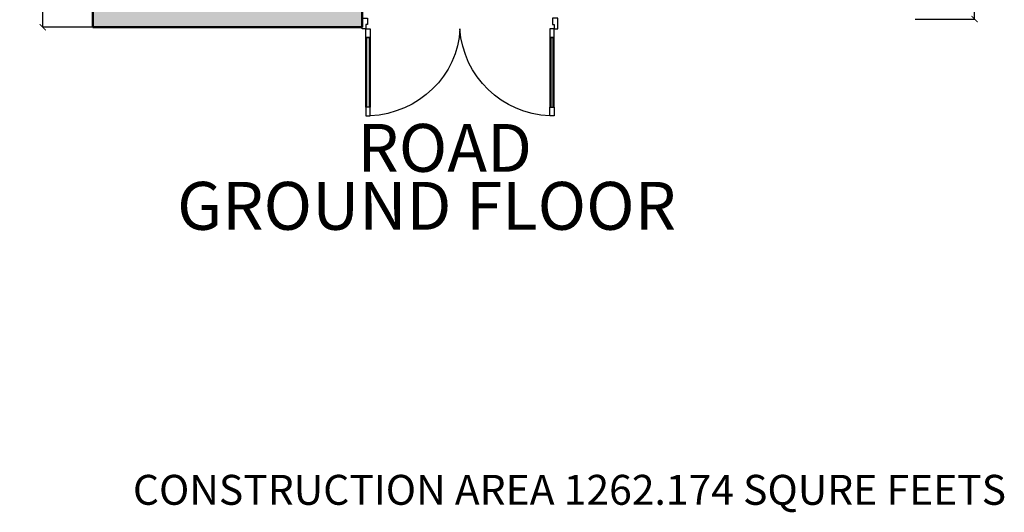
# Model space of a CAD drawing. Units: inches. Extents: x 2278 to 7495, y -71 to 1198.
# Tile 1 of 44: x 2278 to 2761, y 472 to 714. Entities that reach past the tile are written whole.
import ezdxf

# ---------------------------------------------------------------- set-up
doc = ezdxf.new("R2010")
doc.units = ezdxf.units.IN
doc.header["$MEASUREMENT"] = 0
for name, color, linetype, lineweight in [('A-ANNO-DIMS', 2, 'Continuous', 18), ('A-ANNO-TEXT', 7, 'Continuous', 25), ('A-Door', 3, 'Continuous', 25), ('A-Glaz', 4, 'Continuous', 25), ('A-Wall', 7, 'Continuous', 50), ('A-WALL-PATT', 8, 'Continuous', 18)]:
    doc.layers.add(name, color=color, linetype=linetype, lineweight=lineweight)
doc.styles.get("Standard").update_dxf_attribs({"font": 'arial.ttf'})
doc.dimstyles.get("Standard").update_dxf_attribs({"dimtxt": 6, "dimasz": 3, "dimexe": 0.18, "dimexo": 0.0625, "dimgap": 0.09, "dimtad": 0, "dimtih": 1, "dimtoh": 1, "dimdec": 0, "dimzin": 0, "dimdsep": 46, "dimlunit": 3, "dimtxsty": 'Standard', "dimblk": 'ARCHTICK', "dimcen": 0.09, "dimadec": 0, "dimazin": 0, "dimtfac": 1, "dimtdec": 0, "dimtofl": 0, "dimtmove": 0, "dimatfit": 3, "dimfxl": 1, "dimtolj": 1, "dimtzin": 0, "dimarcsym": 0})

# ---------------------------------------------------------------- blocks, each defined once
blk = doc.blocks.new('A$C58286AE3')
for p, q in [((75, 820), (35, 820)), ((35, 820), (35, 180)), ((65, 820), (45, 820)), ((75, 180), (75, 820)), ((75, 180), (35, 180)), ((35, 180), (75, 180)), ((45, 180), (65, 180))]:
    blk.add_line(p, q)
blk.add_lwpolyline([(1725, 180), (1725, 820), (1765, 820), (1765, 180)], close=True)
blk.add_arc((1756.5, 42.1), 858.5, 92.10381, 176.13339)
blk.add_ellipse((70, 105), major_axis=(-772.1, 325.5), ratio=0.94084, start_param=-2.726592, end_param=-1.199193)
at = {"layer": 'A-Door'}
for p, q in [((35, 820), (35, 900)), ((35, 900), (75, 900)), ((75, 820), (35, 820)), ((75, 900), (75, 820)), ((35, 100), (0, 100)), ((0, 100), (0, 0)), ((35, 180), (35, 100)), ((35, 60), (35, 100)), ((35, 100), (75, 100)), ((75, 100), (75, 180)), ((50, 60), (35, 60)), ((50, 50), (50, 60)), ((50, 0), (50, 50)), ((0, 0), (50, 0))]:
    blk.add_line(p, q, dxfattribs=at)
for points in [[(1725, 900), (1725, 820), (1765, 820), (1765, 900)], [(1725, 100), (1725, 180), (1765, 180), (1765, 100)], [(1765, 100), (1800, 100), (1800, 0), (1750, 0), (1750, 50), (1750, 60), (1765, 60)]]:
    blk.add_lwpolyline(points, close=True, dxfattribs=at)
at = {"layer": 'A-Glaz'}
for p, q in [((45, 820), (45, 180)), ((65, 180), (65, 820))]:
    blk.add_line(p, q, dxfattribs=at)
blk.add_lwpolyline([(1735, 180), (1735, 820), (1755, 820), (1755, 180)], close=True, dxfattribs=at)
blk = doc.blocks.new('_ArchTick')
at = {"color": 0, "linetype": 'ByBlock', "const_width": 0.15}
blk.add_lwpolyline([(-0.5, -0.5), (0.5, 0.5)], dxfattribs=at)
blk = doc.blocks.new('*D17')
at = {"layer": 'A-ANNO-DIMS', "color": 0, "lineweight": -2, "transparency": 16777216}
for p, q in [((2313.81, 1163.47), (2289.2, 1163.47)), ((2289.38, 1163.47), (2289.38, 940.12)), ((2289.38, 710.47), (2289.38, 933.81)), ((2313.81, 710.47), (2289.2, 710.47))]:
    blk.add_line(p, q, dxfattribs=at)
at = {"layer": 'Defpoints', "color": 0, "transparency": 16777216}
for p in [(2313.87, 1163.47), (2289.38, 710.47), (2313.87, 710.47)]:
    blk.add_point(p, dxfattribs=at)
at = {"layer": 'A-ANNO-DIMS', "color": 0, "lineweight": -2, "transparency": 16777216, "xscale": 3, "yscale": 3, "zscale": 3}
for p, rotation in [((2289.38, 1163.47), 90), ((2289.38, 710.47), 270)]:
    blk.add_blockref('_ArchTick', p, dxfattribs=dict(at, rotation=rotation))
at = {"layer": 'A-ANNO-DIMS', "color": 0, "transparency": 16777216, "insert": (2289.38, 936.97), "char_height": 6, "attachment_point": 5}
blk.add_mtext('\\A1;37\'-9"', dxfattribs=at)
blk = doc.blocks.new('*D74')
at = {"layer": 'A-ANNO-DIMS', "color": 0, "lineweight": -2, "transparency": 16777216}
for p, q in [((2716.93, 797.47), (2746.3, 797.47)), ((2746.12, 797.47), (2746.12, 759.12)), ((2746.12, 714.47), (2746.12, 752.81)), ((2716.93, 714.47), (2746.3, 714.47))]:
    blk.add_line(p, q, dxfattribs=at)
at = {"layer": 'Defpoints', "color": 0, "transparency": 16777216}
for p in [(2716.87, 797.47), (2716.87, 714.47), (2746.12, 714.47)]:
    blk.add_point(p, dxfattribs=at)
at = {"layer": 'A-ANNO-DIMS', "color": 0, "lineweight": -2, "transparency": 16777216, "xscale": 3, "yscale": 3, "zscale": 3}
for p, rotation in [((2746.12, 797.47), 90), ((2746.12, 714.47), 270)]:
    blk.add_blockref('_ArchTick', p, dxfattribs=dict(at, rotation=rotation))
at = {"layer": 'A-ANNO-DIMS', "color": 0, "transparency": 16777216, "insert": (2746.12, 755.97), "char_height": 6, "attachment_point": 5}
blk.add_mtext('\\A1;6\'-11"', dxfattribs=at)

msp = doc.modelspace()

# ---------------------------------------------------------------- hatches: boundary and pattern name
at = {"layer": 'A-WALL-PATT'}
h = msp.add_hatch(dxfattribs=at)
h.set_pattern_fill('ANSI36', color=256, scale=30)
h.paths.add_polyline_path([(2343.12, 957.47), (2322.87, 957.47), (2322.87, 1029.47), (2351.87, 1029.47), (2351.87, 1034.47), (2322.87, 1034.47), (2322.87, 1154.47), (2339.87, 1154.47), (2339.87, 1163.47), (2313.87, 1163.47), (2313.87, 710.47), (2445.87, 710.47), (2445.87, 719.47), (2322.87, 719.47), (2322.87, 807.47), (2404.87, 807.47), (2404.87, 812.47), (2392.87, 812.47), (2392.87, 881.47), (2387.87, 881.47), (2387.87, 812.47), (2322.87, 812.47), (2322.87, 911.47), (2345.87, 911.47), (2345.87, 916.47), (2322.87, 916.47), (2322.87, 952.47), (2343.12, 952.47)])
h.paths.add_polyline_path([(2451.87, 1163.47), (2411.87, 1163.47), (2411.87, 1154.47), (2428.87, 1154.47), (2428.87, 1034.47), (2428.87, 1029.47), (2433.87, 1029.47), (2433.87, 1154.47), (2451.87, 1154.47)])
h.paths.add_polyline_path([(2558.87, 1163.47), (2523.87, 1163.47), (2523.87, 1154.47), (2541.87, 1154.47), (2541.87, 1034.47), (2475.87, 1034.47), (2475.87, 1029.47), (2541.87, 1029.47), (2541.87, 943.47), (2541.87, 940.13), (2541.87, 876.47), (2493.87, 876.47), (2493.87, 943.47), (2488.87, 943.47), (2488.87, 871.47), (2488.87, 865.74), (2493.88, 865.74), (2493.88, 871.47), (2541.87, 871.47), (2541.87, 805.47), (2546.87, 805.47), (2546.87, 1077.47), (2558.87, 1077.47), (2558.87, 1082.47), (2546.87, 1082.47), (2546.87, 1154.47), (2558.87, 1154.47)])
h.paths.add_polyline_path([(2716.87, 937.97), (2707.87, 937.97), (2707.87, 911.47), (2594.87, 911.47), (2594.87, 906.47), (2707.87, 906.47), (2707.87, 869.47), (2716.87, 869.47)])
h.paths.add_polyline_path([(2716.87, 1163.47), (2689.87, 1163.47), (2689.87, 1154.47), (2707.87, 1154.47), (2707.87, 1041.47), (2594.87, 1041.47), (2594.87, 1036.47), (2707.87, 1036.47), (2707.87, 1009.97), (2716.87, 1009.97)])
h.paths.add_polyline_path([(2617.87, 1163.47), (2582.87, 1163.47), (2582.87, 1154.47), (2594.87, 1154.47), (2594.87, 1082.47), (2588.87, 1082.47), (2588.87, 1077.47), (2599.87, 1077.47), (2599.87, 1154.47), (2617.87, 1154.47)])
h.paths.add_polyline_path([(2716.87, 797.47), (2707.87, 797.47), (2707.87, 760.47), (2663.37, 760.47), (2663.37, 755.47), (2716.87, 755.47)])
h.paths.add_polyline_path([(2591.37, 760.47), (2546.87, 760.47), (2546.87, 763.47), (2541.87, 763.47), (2541.87, 755.47), (2591.37, 755.47)])

# ---------------------------------------------------------------- linework, layer by layer
at = {"layer": 'A-Wall'}
for p, q in [((2313.87, 1163.47), (2313.87, 710.47)), ((2445.87, 710.47), (2445.87, 719.47)), ((2313.87, 710.47), (2445.87, 710.47))]:
    msp.add_line(p, q, dxfattribs=at)

# ---------------------------------------------------------------- block references
at = {"layer": 'A-Door', "xscale": -0.0533333333333331, "yscale": 0.0533333333333331, "zscale": 0.0533333333333331, "rotation": 180}
msp.add_blockref('A$C58286AE3', (2445.87, 714.97), dxfattribs=at)

# ---------------------------------------------------------------- texts
at = {"layer": 'A-ANNO-TEXT'}
for s, height, p in [('ROAD', 23.481, (2443.55, 639.52)), ('GROUND FLOOR', 23.4811, (2355.21, 611.08)), ('CONSTRUCTION AREA 1262.174 SQURE FEETS', 14.6894, (2333.56, 476.15))]:
    msp.add_text(s, height=height, dxfattribs=at).set_placement(p)

# ---------------------------------------------------------------- dimensions: what is measured, and where the dimension line sits
at = {"layer": 'A-ANNO-DIMS'}
for base, p1, p2, override, picture, middle in [((2289.38, 710.47), (2313.87, 1163.47), (2313.87, 710.47), {"dimclrd": 0, "dimclre": 0, "dimclrt": 0}, '*D17', (2289.38, 936.97)), ((2746.12, 714.47), (2716.87, 797.47), (2716.87, 714.47), {"dimdec": 1, "dimlfac": 1, "dimrnd": 0, "dimzin": 1, "dimdsep": 46, "dimlunit": 4, "dimfrac": 2}, '*D74', (2746.12, 755.97))]:
    dim = msp.add_linear_dim(base=base, p1=p1, p2=p2, angle=90, dimstyle='Standard', override=override, dxfattribs=at)
    dim.commit()
    dim.dimension.update_dxf_attribs({"geometry": picture, "text_midpoint": middle})

doc.saveas('drawing.dxf')
